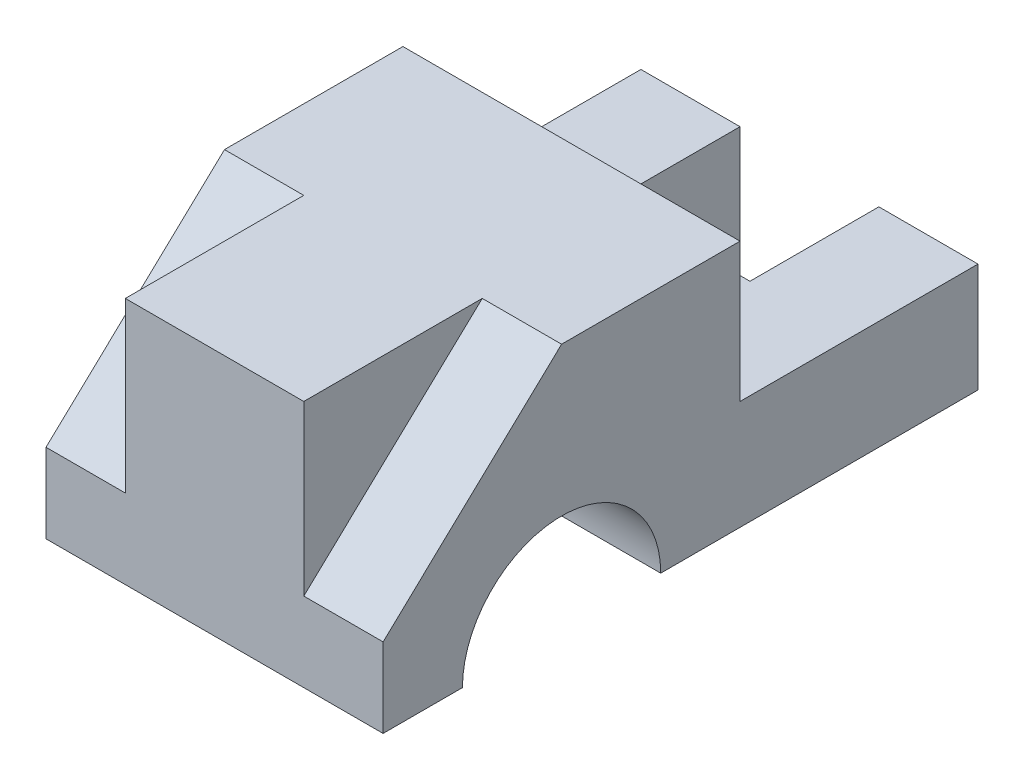
ISO-10303-21;
HEADER;
FILE_DESCRIPTION(('STEP AP214'),'2;1');
FILE_NAME('part.step','',(''),(''),'','','');
FILE_SCHEMA(('AUTOMOTIVE_DESIGN { 1 0 10303 214 1 1 1 1 }'));
ENDSEC;
DATA;
#1=APPLICATION_CONTEXT('core data for automotive mechanical design processes');
#2=APPLICATION_PROTOCOL_DEFINITION('international standard','automotive_design',2000,#1);
#3=PRODUCT_CONTEXT('',#1,'mechanical');
#4=PRODUCT('Part','Part','',(#3));
#5=PRODUCT_RELATED_PRODUCT_CATEGORY('part','',(#4));
#6=PRODUCT_DEFINITION_FORMATION('','',#4);
#7=PRODUCT_DEFINITION_CONTEXT('part definition',#1,'design');
#8=PRODUCT_DEFINITION('design','',#6,#7);
#9=PRODUCT_DEFINITION_SHAPE('','',#8);
#10=(LENGTH_UNIT() NAMED_UNIT(*) SI_UNIT(.MILLI.,.METRE.));
#11=(NAMED_UNIT(*) PLANE_ANGLE_UNIT() SI_UNIT($,.RADIAN.));
#12=(NAMED_UNIT(*) SI_UNIT($,.STERADIAN.) SOLID_ANGLE_UNIT());
#13=UNCERTAINTY_MEASURE_WITH_UNIT(LENGTH_MEASURE(1.E-05),#10,'distance_accuracy_value','');
#14=(GEOMETRIC_REPRESENTATION_CONTEXT(3) GLOBAL_UNCERTAINTY_ASSIGNED_CONTEXT((#13)) GLOBAL_UNIT_ASSIGNED_CONTEXT((#10,
#11,#12)) REPRESENTATION_CONTEXT('',''));
#15=CARTESIAN_POINT('',(0.,0.,0.));
#16=DIRECTION('',(0.,0.,1.));
#17=DIRECTION('',(1.,0.,0.));
#18=AXIS2_PLACEMENT_3D('',#15,#16,#17);
#19=CARTESIAN_POINT('',(34.,12.5,30.));
#20=DIRECTION('',(0.,-1.,0.));
#21=DIRECTION('',(0.,0.,-1.));
#22=AXIS2_PLACEMENT_3D('',#19,#20,#21);
#23=PLANE('',#22);
#24=DIRECTION('',(-1.,0.,0.));
#25=VECTOR('',#24,1.);
#26=CARTESIAN_POINT('',(8.,12.5,12.));
#27=LINE('',#26,#25);
#28=CARTESIAN_POINT('',(8.,12.5,12.));
#29=VERTEX_POINT('',#28);
#30=CARTESIAN_POINT('',(0.,12.5,12.));
#31=VERTEX_POINT('',#30);
#32=EDGE_CURVE('E57',#29,#31,#27,.T.);
#33=ORIENTED_EDGE('',*,*,#32,.F.);
#34=DIRECTION('',(0.,0.,-1.));
#35=VECTOR('',#34,1.);
#36=CARTESIAN_POINT('',(8.,12.5,0.));
#37=LINE('',#36,#35);
#38=CARTESIAN_POINT('',(8.,12.5,30.));
#39=VERTEX_POINT('',#38);
#40=EDGE_CURVE('E161',#39,#29,#37,.T.);
#41=ORIENTED_EDGE('',*,*,#40,.F.);
#42=DIRECTION('',(-1.,0.,0.));
#43=VECTOR('',#42,1.);
#44=CARTESIAN_POINT('',(34.,12.5,30.));
#45=LINE('',#44,#43);
#46=CARTESIAN_POINT('',(26.,12.5,30.));
#47=VERTEX_POINT('',#46);
#48=EDGE_CURVE('E172',#47,#39,#45,.T.);
#49=ORIENTED_EDGE('',*,*,#48,.F.);
#50=DIRECTION('',(0.,0.,1.));
#51=VECTOR('',#50,1.);
#52=CARTESIAN_POINT('',(26.,12.5,0.));
#53=LINE('',#52,#51);
#54=CARTESIAN_POINT('',(26.,12.5,12.));
#55=VERTEX_POINT('',#54);
#56=EDGE_CURVE('E183',#55,#47,#53,.T.);
#57=ORIENTED_EDGE('',*,*,#56,.F.);
#58=DIRECTION('',(1.,0.,0.));
#59=VECTOR('',#58,1.);
#60=CARTESIAN_POINT('',(26.,12.5,12.));
#61=LINE('',#60,#59);
#62=CARTESIAN_POINT('',(34.,12.5,12.));
#63=VERTEX_POINT('',#62);
#64=EDGE_CURVE('E189',#55,#63,#61,.T.);
#65=ORIENTED_EDGE('',*,*,#64,.T.);
#66=DIRECTION('',(0.,0.,1.));
#67=VECTOR('',#66,1.);
#68=CARTESIAN_POINT('',(34.,12.5,30.));
#69=LINE('',#68,#67);
#70=CARTESIAN_POINT('',(34.,12.5,-6.));
#71=VERTEX_POINT('',#70);
#72=EDGE_CURVE('E245',#71,#63,#69,.T.);
#73=ORIENTED_EDGE('',*,*,#72,.F.);
#74=DIRECTION('',(1.,0.,0.));
#75=VECTOR('',#74,1.);
#76=CARTESIAN_POINT('',(0.,12.5,-6.));
#77=LINE('',#76,#75);
#78=CARTESIAN_POINT('',(0.,12.5,-6.));
#79=VERTEX_POINT('',#78);
#80=EDGE_CURVE('E218',#79,#71,#77,.T.);
#81=ORIENTED_EDGE('',*,*,#80,.F.);
#82=DIRECTION('',(0.,0.,1.));
#83=VECTOR('',#82,1.);
#84=CARTESIAN_POINT('',(0.,12.5,30.));
#85=LINE('',#84,#83);
#86=EDGE_CURVE('E256',#79,#31,#85,.T.);
#87=ORIENTED_EDGE('',*,*,#86,.T.);
#88=EDGE_LOOP('',(#33,#41,#49,#57,#65,#73,#81,#87));
#89=FACE_BOUND('',#88,.T.);
#90=ADVANCED_FACE('F41',(#89),#23,.F.);
#91=CARTESIAN_POINT('',(34.,12.5,30.));
#92=DIRECTION('',(0.,0.,-1.));
#93=DIRECTION('',(-1.,0.,0.));
#94=AXIS2_PLACEMENT_3D('',#91,#92,#93);
#95=PLANE('',#94);
#96=DIRECTION('',(-1.,0.,0.));
#97=VECTOR('',#96,1.);
#98=CARTESIAN_POINT('',(8.,-4.5,30.));
#99=LINE('',#98,#97);
#100=CARTESIAN_POINT('',(8.,-4.5,30.));
#101=VERTEX_POINT('',#100);
#102=CARTESIAN_POINT('',(0.,-4.5,30.));
#103=VERTEX_POINT('',#102);
#104=EDGE_CURVE('E155',#101,#103,#99,.T.);
#105=ORIENTED_EDGE('',*,*,#104,.T.);
#106=DIRECTION('',(0.,-1.,0.));
#107=VECTOR('',#106,1.);
#108=CARTESIAN_POINT('',(0.,12.5,30.));
#109=LINE('',#108,#107);
#110=CARTESIAN_POINT('',(0.,-12.5,30.));
#111=VERTEX_POINT('',#110);
#112=EDGE_CURVE('E261',#103,#111,#109,.T.);
#113=ORIENTED_EDGE('',*,*,#112,.T.);
#114=DIRECTION('',(-1.,0.,0.));
#115=VECTOR('',#114,1.);
#116=CARTESIAN_POINT('',(34.,-12.5,30.));
#117=LINE('',#116,#115);
#118=CARTESIAN_POINT('',(34.,-12.5,30.));
#119=VERTEX_POINT('',#118);
#120=EDGE_CURVE('E267',#119,#111,#117,.T.);
#121=ORIENTED_EDGE('',*,*,#120,.F.);
#122=DIRECTION('',(0.,-1.,0.));
#123=VECTOR('',#122,1.);
#124=CARTESIAN_POINT('',(34.,12.5,30.));
#125=LINE('',#124,#123);
#126=CARTESIAN_POINT('',(34.,-4.50000000000001,30.));
#127=VERTEX_POINT('',#126);
#128=EDGE_CURVE('E247',#127,#119,#125,.T.);
#129=ORIENTED_EDGE('',*,*,#128,.F.);
#130=DIRECTION('',(1.,0.,0.));
#131=VECTOR('',#130,1.);
#132=CARTESIAN_POINT('',(26.,-4.5,30.));
#133=LINE('',#132,#131);
#134=CARTESIAN_POINT('',(26.,-4.5,30.));
#135=VERTEX_POINT('',#134);
#136=EDGE_CURVE('E63',#135,#127,#133,.T.);
#137=ORIENTED_EDGE('',*,*,#136,.F.);
#138=DIRECTION('',(0.,-1.,0.));
#139=VECTOR('',#138,1.);
#140=CARTESIAN_POINT('',(26.,0.,30.));
#141=LINE('',#140,#139);
#142=EDGE_CURVE('E177',#47,#135,#141,.T.);
#143=ORIENTED_EDGE('',*,*,#142,.F.);
#144=ORIENTED_EDGE('',*,*,#48,.T.);
#145=DIRECTION('',(0.,1.,0.));
#146=VECTOR('',#145,1.);
#147=CARTESIAN_POINT('',(8.,0.,30.));
#148=LINE('',#147,#146);
#149=EDGE_CURVE('E164',#101,#39,#148,.T.);
#150=ORIENTED_EDGE('',*,*,#149,.F.);
#151=EDGE_LOOP('',(#105,#113,#121,#129,#137,#143,#144,#150));
#152=FACE_BOUND('',#151,.T.);
#153=ADVANCED_FACE('F166',(#152),#95,.F.);
#154=CARTESIAN_POINT('',(0.,0.,0.));
#155=DIRECTION('',(1.,0.,0.));
#156=DIRECTION('',(0.,0.,-1.));
#157=AXIS2_PLACEMENT_3D('',#154,#155,#156);
#158=PLANE('',#157);
#159=DIRECTION('',(0.,0.686623532963717,-0.727013152549817));
#160=VECTOR('',#159,1.);
#161=CARTESIAN_POINT('',(0.,12.5970636215334,11.8972267536705));
#162=LINE('',#161,#160);
#163=EDGE_CURVE('E160',#103,#31,#162,.T.);
#164=ORIENTED_EDGE('',*,*,#163,.T.);
#165=ORIENTED_EDGE('',*,*,#86,.F.);
#166=DIRECTION('',(0.,-1.,0.));
#167=VECTOR('',#166,1.);
#168=CARTESIAN_POINT('',(0.,12.5,-6.));
#169=LINE('',#168,#167);
#170=CARTESIAN_POINT('',(0.,-1.50000000000001,-6.));
#171=VERTEX_POINT('',#170);
#172=EDGE_CURVE('E215',#79,#171,#169,.T.);
#173=ORIENTED_EDGE('',*,*,#172,.T.);
#174=DIRECTION('',(0.,0.,-1.));
#175=VECTOR('',#174,1.);
#176=CARTESIAN_POINT('',(0.,-1.5,-30.));
#177=LINE('',#176,#175);
#178=CARTESIAN_POINT('',(0.,-1.5,-30.));
#179=VERTEX_POINT('',#178);
#180=EDGE_CURVE('E214',#171,#179,#177,.T.);
#181=ORIENTED_EDGE('',*,*,#180,.T.);
#182=DIRECTION('',(0.,1.,0.));
#183=VECTOR('',#182,1.);
#184=CARTESIAN_POINT('',(0.,12.5,-30.));
#185=LINE('',#184,#183);
#186=CARTESIAN_POINT('',(0.,-12.5,-30.));
#187=VERTEX_POINT('',#186);
#188=EDGE_CURVE('E228',#187,#179,#185,.T.);
#189=ORIENTED_EDGE('',*,*,#188,.F.);
#190=DIRECTION('',(0.,0.,-1.));
#191=VECTOR('',#190,1.);
#192=CARTESIAN_POINT('',(0.,-12.5,30.));
#193=LINE('',#192,#191);
#194=CARTESIAN_POINT('',(0.,-12.5,1.99999999999999));
#195=VERTEX_POINT('',#194);
#196=EDGE_CURVE('E263',#195,#187,#193,.T.);
#197=ORIENTED_EDGE('',*,*,#196,.F.);
#198=CARTESIAN_POINT('',(0.,-12.5,12.));
#199=DIRECTION('',(1.,0.,0.));
#200=DIRECTION('',(0.,0.,1.));
#201=AXIS2_PLACEMENT_3D('',#198,#199,#200);
#202=CIRCLE('',#201,10.);
#203=CARTESIAN_POINT('',(0.,-12.5,22.));
#204=VERTEX_POINT('',#203);
#205=EDGE_CURVE('E232',#195,#204,#202,.T.);
#206=ORIENTED_EDGE('',*,*,#205,.T.);
#207=EDGE_CURVE('E248',#111,#204,#193,.T.);
#208=ORIENTED_EDGE('',*,*,#207,.F.);
#209=ORIENTED_EDGE('',*,*,#112,.F.);
#210=EDGE_LOOP('',(#164,#165,#173,#181,#189,#197,#206,#208,#209));
#211=FACE_BOUND('',#210,.T.);
#212=ADVANCED_FACE('F301',(#211),#158,.F.);
#213=CARTESIAN_POINT('',(34.,12.5,-30.));
#214=DIRECTION('',(0.,0.,1.));
#215=DIRECTION('',(1.,0.,0.));
#216=AXIS2_PLACEMENT_3D('',#213,#214,#215);
#217=PLANE('',#216);
#218=DIRECTION('',(1.,0.,0.));
#219=VECTOR('',#218,1.);
#220=CARTESIAN_POINT('',(0.,-1.5,-30.));
#221=LINE('',#220,#219);
#222=CARTESIAN_POINT('',(10.,-1.5,-30.));
#223=VERTEX_POINT('',#222);
#224=EDGE_CURVE('E226',#179,#223,#221,.T.);
#225=ORIENTED_EDGE('',*,*,#224,.T.);
#226=DIRECTION('',(0.,1.,0.));
#227=VECTOR('',#226,1.);
#228=CARTESIAN_POINT('',(10.,-21.5,-30.));
#229=LINE('',#228,#227);
#230=CARTESIAN_POINT('',(10.,-12.5,-30.));
#231=VERTEX_POINT('',#230);
#232=EDGE_CURVE('E191',#231,#223,#229,.T.);
#233=ORIENTED_EDGE('',*,*,#232,.F.);
#234=DIRECTION('',(-1.,0.,0.));
#235=VECTOR('',#234,1.);
#236=CARTESIAN_POINT('',(34.,-12.5,-30.));
#237=LINE('',#236,#235);
#238=EDGE_CURVE('E254',#231,#187,#237,.T.);
#239=ORIENTED_EDGE('',*,*,#238,.T.);
#240=ORIENTED_EDGE('',*,*,#188,.T.);
#241=EDGE_LOOP('',(#225,#233,#239,#240));
#242=FACE_BOUND('',#241,.T.);
#243=ADVANCED_FACE('F299',(#242),#217,.F.);
#244=CARTESIAN_POINT('',(34.,-12.5,30.));
#245=DIRECTION('',(0.,1.,0.));
#246=DIRECTION('',(0.,0.,1.));
#247=AXIS2_PLACEMENT_3D('',#244,#245,#246);
#248=PLANE('',#247);
#249=ORIENTED_EDGE('',*,*,#207,.T.);
#250=DIRECTION('',(1.,0.,0.));
#251=VECTOR('',#250,1.);
#252=CARTESIAN_POINT('',(0.,-12.5,22.));
#253=LINE('',#252,#251);
#254=CARTESIAN_POINT('',(34.,-12.5,22.));
#255=VERTEX_POINT('',#254);
#256=EDGE_CURVE('E240',#204,#255,#253,.T.);
#257=ORIENTED_EDGE('',*,*,#256,.T.);
#258=DIRECTION('',(0.,0.,-1.));
#259=VECTOR('',#258,1.);
#260=CARTESIAN_POINT('',(34.,-12.5,30.));
#261=LINE('',#260,#259);
#262=EDGE_CURVE('E252',#119,#255,#261,.T.);
#263=ORIENTED_EDGE('',*,*,#262,.F.);
#264=ORIENTED_EDGE('',*,*,#120,.T.);
#265=EDGE_LOOP('',(#249,#257,#263,#264));
#266=FACE_BOUND('',#265,.T.);
#267=ADVANCED_FACE('F317',(#266),#248,.F.);
#268=CARTESIAN_POINT('',(34.,-12.5,-30.));
#269=VERTEX_POINT('',#268);
#270=CARTESIAN_POINT('',(24.,-12.5,-30.));
#271=VERTEX_POINT('',#270);
#272=EDGE_CURVE('E266',#269,#271,#237,.T.);
#273=ORIENTED_EDGE('',*,*,#272,.T.);
#274=DIRECTION('',(0.,1.,0.));
#275=VECTOR('',#274,1.);
#276=CARTESIAN_POINT('',(24.,-21.5,-30.));
#277=LINE('',#276,#275);
#278=CARTESIAN_POINT('',(24.,-1.5,-30.));
#279=VERTEX_POINT('',#278);
#280=EDGE_CURVE('E198',#271,#279,#277,.T.);
#281=ORIENTED_EDGE('',*,*,#280,.T.);
#282=CARTESIAN_POINT('',(34.,-1.5,-30.));
#283=VERTEX_POINT('',#282);
#284=EDGE_CURVE('E230',#279,#283,#221,.T.);
#285=ORIENTED_EDGE('',*,*,#284,.T.);
#286=DIRECTION('',(0.,1.,0.));
#287=VECTOR('',#286,1.);
#288=CARTESIAN_POINT('',(34.,12.5,-30.));
#289=LINE('',#288,#287);
#290=EDGE_CURVE('E242',#269,#283,#289,.T.);
#291=ORIENTED_EDGE('',*,*,#290,.F.);
#292=EDGE_LOOP('',(#273,#281,#285,#291));
#293=FACE_BOUND('',#292,.T.);
#294=ADVANCED_FACE('F43',(#293),#217,.F.);
#295=ORIENTED_EDGE('',*,*,#238,.F.);
#296=DIRECTION('',(0.,0.,1.));
#297=VECTOR('',#296,1.);
#298=CARTESIAN_POINT('',(10.,-12.5,30.));
#299=LINE('',#298,#297);
#300=CARTESIAN_POINT('',(10.,-12.5,-17.));
#301=VERTEX_POINT('',#300);
#302=EDGE_CURVE('E208',#231,#301,#299,.T.);
#303=ORIENTED_EDGE('',*,*,#302,.T.);
#304=DIRECTION('',(1.,0.,0.));
#305=VECTOR('',#304,1.);
#306=CARTESIAN_POINT('',(34.,-12.5,-17.));
#307=LINE('',#306,#305);
#308=CARTESIAN_POINT('',(24.,-12.5,-17.));
#309=VERTEX_POINT('',#308);
#310=EDGE_CURVE('E194',#301,#309,#307,.T.);
#311=ORIENTED_EDGE('',*,*,#310,.T.);
#312=DIRECTION('',(0.,0.,-1.));
#313=VECTOR('',#312,1.);
#314=CARTESIAN_POINT('',(24.,-12.5,30.));
#315=LINE('',#314,#313);
#316=EDGE_CURVE('E202',#309,#271,#315,.T.);
#317=ORIENTED_EDGE('',*,*,#316,.T.);
#318=ORIENTED_EDGE('',*,*,#272,.F.);
#319=CARTESIAN_POINT('',(34.,-12.5,1.99999999999999));
#320=VERTEX_POINT('',#319);
#321=EDGE_CURVE('E253',#320,#269,#261,.T.);
#322=ORIENTED_EDGE('',*,*,#321,.F.);
#323=DIRECTION('',(1.,0.,0.));
#324=VECTOR('',#323,1.);
#325=CARTESIAN_POINT('',(0.,-12.5,1.99999999999999));
#326=LINE('',#325,#324);
#327=EDGE_CURVE('E224',#195,#320,#326,.T.);
#328=ORIENTED_EDGE('',*,*,#327,.F.);
#329=ORIENTED_EDGE('',*,*,#196,.T.);
#330=EDGE_LOOP('',(#295,#303,#311,#317,#318,#322,#328,#329));
#331=FACE_BOUND('',#330,.T.);
#332=ADVANCED_FACE('F286',(#331),#248,.F.);
#333=CARTESIAN_POINT('',(34.,0.,0.));
#334=DIRECTION('',(1.,0.,0.));
#335=DIRECTION('',(0.,0.,-1.));
#336=AXIS2_PLACEMENT_3D('',#333,#334,#335);
#337=PLANE('',#336);
#338=DIRECTION('',(0.,0.686623532963716,-0.727013152549818));
#339=VECTOR('',#338,1.);
#340=CARTESIAN_POINT('',(34.,12.5970636215334,11.8972267536705));
#341=LINE('',#340,#339);
#342=EDGE_CURVE('E180',#127,#63,#341,.T.);
#343=ORIENTED_EDGE('',*,*,#342,.F.);
#344=ORIENTED_EDGE('',*,*,#128,.T.);
#345=ORIENTED_EDGE('',*,*,#262,.T.);
#346=CARTESIAN_POINT('',(34.,-12.5,12.));
#347=DIRECTION('',(1.,0.,0.));
#348=DIRECTION('',(0.,0.,1.));
#349=AXIS2_PLACEMENT_3D('',#346,#347,#348);
#350=CIRCLE('',#349,10.);
#351=EDGE_CURVE('E211',#320,#255,#350,.T.);
#352=ORIENTED_EDGE('',*,*,#351,.F.);
#353=ORIENTED_EDGE('',*,*,#321,.T.);
#354=ORIENTED_EDGE('',*,*,#290,.T.);
#355=DIRECTION('',(0.,0.,-1.));
#356=VECTOR('',#355,1.);
#357=CARTESIAN_POINT('',(34.,-1.5,-30.));
#358=LINE('',#357,#356);
#359=CARTESIAN_POINT('',(34.,-1.50000000000001,-6.));
#360=VERTEX_POINT('',#359);
#361=EDGE_CURVE('E216',#360,#283,#358,.T.);
#362=ORIENTED_EDGE('',*,*,#361,.F.);
#363=DIRECTION('',(0.,-1.,0.));
#364=VECTOR('',#363,1.);
#365=CARTESIAN_POINT('',(34.,12.5,-6.));
#366=LINE('',#365,#364);
#367=EDGE_CURVE('E219',#71,#360,#366,.T.);
#368=ORIENTED_EDGE('',*,*,#367,.F.);
#369=ORIENTED_EDGE('',*,*,#72,.T.);
#370=EDGE_LOOP('',(#343,#344,#345,#352,#353,#354,#362,#368,#369));
#371=FACE_BOUND('',#370,.T.);
#372=ADVANCED_FACE('F311',(#371),#337,.T.);
#373=CARTESIAN_POINT('',(0.,-12.5,12.));
#374=DIRECTION('',(1.,0.,0.));
#375=DIRECTION('',(0.,0.,-1.));
#376=AXIS2_PLACEMENT_3D('',#373,#374,#375);
#377=CYLINDRICAL_SURFACE('',#376,10.);
#378=ORIENTED_EDGE('',*,*,#351,.T.);
#379=ORIENTED_EDGE('',*,*,#256,.F.);
#380=ORIENTED_EDGE('',*,*,#205,.F.);
#381=ORIENTED_EDGE('',*,*,#327,.T.);
#382=EDGE_LOOP('',(#378,#379,#380,#381));
#383=FACE_BOUND('',#382,.T.);
#384=ADVANCED_FACE('F320',(#383),#377,.F.);
#385=CARTESIAN_POINT('',(0.,-1.5,-30.));
#386=DIRECTION('',(0.,-1.,0.));
#387=DIRECTION('',(0.,0.,-1.));
#388=AXIS2_PLACEMENT_3D('',#385,#386,#387);
#389=PLANE('',#388);
#390=DIRECTION('',(-1.,0.,0.));
#391=VECTOR('',#390,1.);
#392=CARTESIAN_POINT('',(0.,-1.50000000000001,-17.));
#393=LINE('',#392,#391);
#394=CARTESIAN_POINT('',(24.,-1.5,-17.));
#395=VERTEX_POINT('',#394);
#396=CARTESIAN_POINT('',(10.,-1.50000000000001,-17.));
#397=VERTEX_POINT('',#396);
#398=EDGE_CURVE('E272',#395,#397,#393,.T.);
#399=ORIENTED_EDGE('',*,*,#398,.T.);
#400=DIRECTION('',(0.,0.,-1.));
#401=VECTOR('',#400,1.);
#402=CARTESIAN_POINT('',(10.,-1.5,-30.));
#403=LINE('',#402,#401);
#404=EDGE_CURVE('E11',#397,#223,#403,.T.);
#405=ORIENTED_EDGE('',*,*,#404,.T.);
#406=ORIENTED_EDGE('',*,*,#224,.F.);
#407=ORIENTED_EDGE('',*,*,#180,.F.);
#408=DIRECTION('',(1.,0.,0.));
#409=VECTOR('',#408,1.);
#410=CARTESIAN_POINT('',(0.,-1.50000000000001,-6.));
#411=LINE('',#410,#409);
#412=EDGE_CURVE('E233',#171,#360,#411,.T.);
#413=ORIENTED_EDGE('',*,*,#412,.T.);
#414=ORIENTED_EDGE('',*,*,#361,.T.);
#415=ORIENTED_EDGE('',*,*,#284,.F.);
#416=DIRECTION('',(0.,0.,1.));
#417=VECTOR('',#416,1.);
#418=CARTESIAN_POINT('',(24.,-1.5,-30.));
#419=LINE('',#418,#417);
#420=EDGE_CURVE('E47',#279,#395,#419,.T.);
#421=ORIENTED_EDGE('',*,*,#420,.T.);
#422=EDGE_LOOP('',(#399,#405,#406,#407,#413,#414,#415,#421));
#423=FACE_BOUND('',#422,.T.);
#424=ADVANCED_FACE('F279',(#423),#389,.F.);
#425=CARTESIAN_POINT('',(0.,12.5,-6.));
#426=DIRECTION('',(0.,0.,1.));
#427=DIRECTION('',(1.,0.,0.));
#428=AXIS2_PLACEMENT_3D('',#425,#426,#427);
#429=PLANE('',#428);
#430=ORIENTED_EDGE('',*,*,#367,.T.);
#431=ORIENTED_EDGE('',*,*,#412,.F.);
#432=ORIENTED_EDGE('',*,*,#172,.F.);
#433=ORIENTED_EDGE('',*,*,#80,.T.);
#434=EDGE_LOOP('',(#430,#431,#432,#433));
#435=FACE_BOUND('',#434,.T.);
#436=ADVANCED_FACE('F307',(#435),#429,.F.);
#437=CARTESIAN_POINT('',(10.,-21.5,-30.));
#438=DIRECTION('',(-1.,0.,0.));
#439=DIRECTION('',(0.,0.,1.));
#440=AXIS2_PLACEMENT_3D('',#437,#438,#439);
#441=PLANE('',#440);
#442=ORIENTED_EDGE('',*,*,#232,.T.);
#443=ORIENTED_EDGE('',*,*,#404,.F.);
#444=DIRECTION('',(0.,1.,0.));
#445=VECTOR('',#444,1.);
#446=CARTESIAN_POINT('',(10.,-21.5,-17.));
#447=LINE('',#446,#445);
#448=EDGE_CURVE('E193',#301,#397,#447,.T.);
#449=ORIENTED_EDGE('',*,*,#448,.F.);
#450=ORIENTED_EDGE('',*,*,#302,.F.);
#451=EDGE_LOOP('',(#442,#443,#449,#450));
#452=FACE_BOUND('',#451,.T.);
#453=ADVANCED_FACE('F293',(#452),#441,.F.);
#454=CARTESIAN_POINT('',(24.,-21.5,-30.));
#455=DIRECTION('',(1.,0.,0.));
#456=DIRECTION('',(0.,0.,-1.));
#457=AXIS2_PLACEMENT_3D('',#454,#455,#456);
#458=PLANE('',#457);
#459=DIRECTION('',(0.,1.,0.));
#460=VECTOR('',#459,1.);
#461=CARTESIAN_POINT('',(24.,-21.5,-17.));
#462=LINE('',#461,#460);
#463=EDGE_CURVE('E200',#309,#395,#462,.T.);
#464=ORIENTED_EDGE('',*,*,#463,.T.);
#465=ORIENTED_EDGE('',*,*,#420,.F.);
#466=ORIENTED_EDGE('',*,*,#280,.F.);
#467=ORIENTED_EDGE('',*,*,#316,.F.);
#468=EDGE_LOOP('',(#464,#465,#466,#467));
#469=FACE_BOUND('',#468,.T.);
#470=ADVANCED_FACE('F278',(#469),#458,.F.);
#471=CARTESIAN_POINT('',(10.,-21.5,-17.));
#472=DIRECTION('',(0.,0.,1.));
#473=DIRECTION('',(1.,0.,0.));
#474=AXIS2_PLACEMENT_3D('',#471,#472,#473);
#475=PLANE('',#474);
#476=ORIENTED_EDGE('',*,*,#448,.T.);
#477=ORIENTED_EDGE('',*,*,#398,.F.);
#478=ORIENTED_EDGE('',*,*,#463,.F.);
#479=ORIENTED_EDGE('',*,*,#310,.F.);
#480=EDGE_LOOP('',(#476,#477,#478,#479));
#481=FACE_BOUND('',#480,.T.);
#482=ADVANCED_FACE('F292',(#481),#475,.F.);
#483=CARTESIAN_POINT('',(26.,12.5970636215334,11.8972267536705));
#484=DIRECTION('',(0.,-0.727013152549818,-0.686623532963716));
#485=DIRECTION('',(0.,0.686623532963716,-0.727013152549818));
#486=AXIS2_PLACEMENT_3D('',#483,#484,#485);
#487=PLANE('',#486);
#488=ORIENTED_EDGE('',*,*,#342,.T.);
#489=ORIENTED_EDGE('',*,*,#64,.F.);
#490=DIRECTION('',(0.,0.686623532963716,-0.727013152549818));
#491=VECTOR('',#490,1.);
#492=CARTESIAN_POINT('',(26.,12.5970636215334,11.8972267536705));
#493=LINE('',#492,#491);
#494=EDGE_CURVE('E185',#135,#55,#493,.T.);
#495=ORIENTED_EDGE('',*,*,#494,.F.);
#496=ORIENTED_EDGE('',*,*,#136,.T.);
#497=EDGE_LOOP('',(#488,#489,#495,#496));
#498=FACE_BOUND('',#497,.T.);
#499=ADVANCED_FACE('F323',(#498),#487,.F.);
#500=CARTESIAN_POINT('',(26.,0.,0.));
#501=DIRECTION('',(1.,0.,0.));
#502=DIRECTION('',(0.,0.,-1.));
#503=AXIS2_PLACEMENT_3D('',#500,#501,#502);
#504=PLANE('',#503);
#505=ORIENTED_EDGE('',*,*,#142,.T.);
#506=ORIENTED_EDGE('',*,*,#494,.T.);
#507=ORIENTED_EDGE('',*,*,#56,.T.);
#508=EDGE_LOOP('',(#505,#506,#507));
#509=FACE_BOUND('',#508,.T.);
#510=ADVANCED_FACE('F330',(#509),#504,.T.);
#511=CARTESIAN_POINT('',(8.,12.5970636215334,11.8972267536705));
#512=DIRECTION('',(0.,0.727013152549817,0.686623532963717));
#513=DIRECTION('',(0.,-0.686623532963717,0.727013152549817));
#514=AXIS2_PLACEMENT_3D('',#511,#512,#513);
#515=PLANE('',#514);
#516=ORIENTED_EDGE('',*,*,#163,.F.);
#517=ORIENTED_EDGE('',*,*,#104,.F.);
#518=DIRECTION('',(0.,0.686623532963717,-0.727013152549817));
#519=VECTOR('',#518,1.);
#520=CARTESIAN_POINT('',(8.,12.5970636215334,11.8972267536705));
#521=LINE('',#520,#519);
#522=EDGE_CURVE('E154',#101,#29,#521,.T.);
#523=ORIENTED_EDGE('',*,*,#522,.T.);
#524=ORIENTED_EDGE('',*,*,#32,.T.);
#525=EDGE_LOOP('',(#516,#517,#523,#524));
#526=FACE_BOUND('',#525,.T.);
#527=ADVANCED_FACE('F152',(#526),#515,.T.);
#528=CARTESIAN_POINT('',(8.,0.,0.));
#529=DIRECTION('',(-1.,0.,0.));
#530=DIRECTION('',(0.,0.,1.));
#531=AXIS2_PLACEMENT_3D('',#528,#529,#530);
#532=PLANE('',#531);
#533=ORIENTED_EDGE('',*,*,#522,.F.);
#534=ORIENTED_EDGE('',*,*,#149,.T.);
#535=ORIENTED_EDGE('',*,*,#40,.T.);
#536=EDGE_LOOP('',(#533,#534,#535));
#537=FACE_BOUND('',#536,.T.);
#538=ADVANCED_FACE('F163',(#537),#532,.T.);
#539=CLOSED_SHELL('',(#90,#153,#212,#243,#267,#294,#332,#372,#384,#424,#436,#453,#470,#482,#499,
#510,#527,#538));
#540=MANIFOLD_SOLID_BREP('B2',#539);
#541=ADVANCED_BREP_SHAPE_REPRESENTATION('',(#18,#540),#14);
#542=SHAPE_DEFINITION_REPRESENTATION(#9,#541);
ENDSEC;
END-ISO-10303-21;
